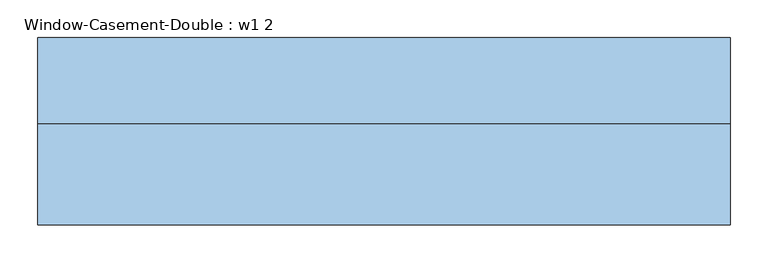
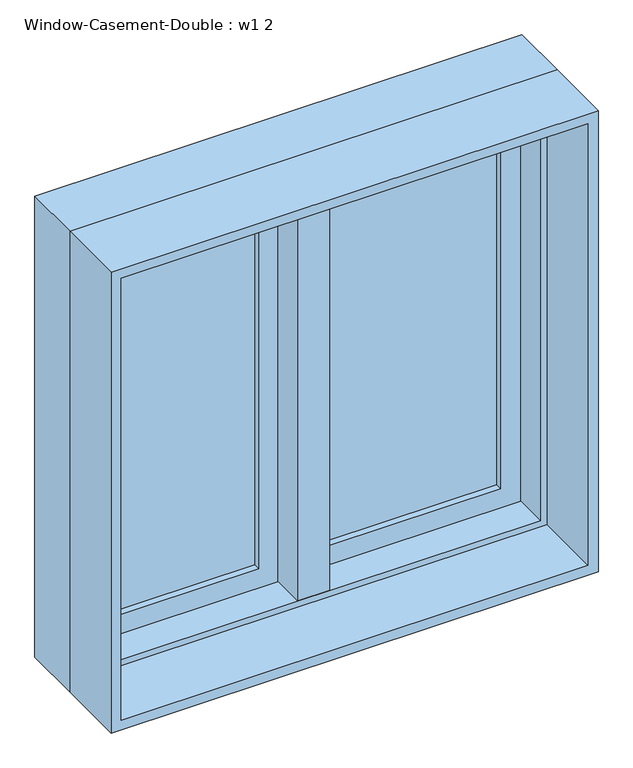
"""IFC4 building model written with IfcOpenShell, lengths in millimetres: window geometry, Window-Casement-Double : w1 2."""

from ifc_helpers import new_model, si_unit, frame, origin, place, context, project, spatial, polyline, outline, extrude, faceted_brep, source, transform, mapped, element, save


def window_casement_double_w1_2_90de19e9(model_context):
    return source(origin(), model_context, "Body", "SolidModel", [
        faceted_brep([(9.525, 133.35, 1816.1), (-9.525, 133.35, 1816.1), (-9.525, 82.55, 1816.1), (9.525, 82.55, 1816.1), (9.525, 133.35, 927.1), (9.525, 82.55, 927.1), (-9.525, 82.55, 927.1), (-9.525, 133.35, 927.1), (-9.525, 82.55, 946.15), (-9.525, 82.55, 1797.05), (-30.1625, 82.55, 946.15), (-30.1625, 82.55, 1797.05), (-30.1625, 19.05, 946.15), (-30.1625, 19.05, 1797.05), (30.1625, 19.05, 946.15), (30.1625, 19.05, 1797.05), (30.1625, 82.55, 946.15), (30.1625, 82.55, 1797.05), (9.525, 82.55, 946.15), (9.525, 82.55, 1797.05)], [[[0, 1, 2, 3]], [[4, 5, 6, 7]], [[1, 0, 4, 7]], [[2, 1, 7, 6, 8, 9]], [[9, 8, 10, 11]], [[11, 10, 12, 13]], [[13, 12, 14, 15]], [[15, 14, 16, 17]], [[17, 16, 18, 19]], [[0, 3, 19, 18, 5, 4]], [[18, 8, 6, 5]], [[9, 19, 3, 2]], [[8, 18, 16, 14, 12, 10]], [[19, 9, 11, 13, 15, 17]]]),
        extrude(outline(polyline([(-66.675, 114.3), (-66.675, 107.95), (-387.35, 107.95), (-387.35, 114.3), (-66.675, 114.3)])), frame((0.0, 0.0, 984.25), z_axis=(0.0, 0.0, 1.0), x_axis=(1.0, 0.0, 0.0)), (0.0, 0.0, 1.0), 774.7),
        extrude(outline(polyline([(-387.35, 95.25), (-387.35, 101.6), (-66.675, 101.6), (-66.675, 95.25), (-387.35, 95.25)])), frame((0.0, 0.0, 984.25), z_axis=(0.0, 0.0, 1.0), x_axis=(1.0, 0.0, 0.0)), (0.0, 0.0, 1.0), 774.7),
        extrude(outline(polyline([(387.35, 114.3), (387.35, 107.95), (66.675, 107.95), (66.675, 114.3), (387.35, 114.3)])), frame((0.0, 0.0, 984.25), z_axis=(0.0, 0.0, 1.0), x_axis=(1.0, 0.0, 0.0)), (0.0, 0.0, 1.0), 774.7),
        extrude(outline(polyline([(66.675, 95.25), (66.675, 101.6), (387.35, 101.6), (387.35, 95.25), (66.675, 95.25)])), frame((0.0, 0.0, 984.25), z_axis=(0.0, 0.0, 1.0), x_axis=(1.0, 0.0, 0.0)), (0.0, 0.0, 1.0), 774.7),
        extrude(outline(polyline([(1816.1, -444.5), (927.1, -444.5), (927.1, -9.525), (1816.1, -9.525), (1816.1, -444.5)]), holes=[polyline([(1758.95, -66.675), (984.25, -66.675), (984.25, -387.35), (1758.95, -387.35), (1758.95, -66.675)])]), frame((0.0, 82.55, 0.0), z_axis=(0.0, 1.0, 0.0), x_axis=(0.0, 0.0, 1.0)), (0.0, 0.0, 1.0), 44.45),
        extrude(outline(polyline([(927.1, 444.5), (1816.1, 444.5), (1816.1, 9.525), (927.1, 9.525), (927.1, 444.5)]), holes=[polyline([(984.25, 66.675), (1758.95, 66.675), (1758.95, 387.35), (984.25, 387.35), (984.25, 66.675)])]), frame((0.0, 82.55, 0.0), z_axis=(0.0, 1.0, 0.0), x_axis=(0.0, 0.0, 1.0)), (0.0, 0.0, 1.0), 44.45),
        extrude(outline(polyline([(1828.8, -457.2), (914.4, -457.2), (914.4, 457.2), (1828.8, 457.2), (1828.8, -457.2)]), holes=[polyline([(1809.75, 438.15), (933.45, 438.15), (933.45, -438.15), (1809.75, -438.15), (1809.75, 438.15)])]), frame((0.0, -114.3, 0.0), z_axis=(0.0, 1.0, 0.0), x_axis=(0.0, 0.0, 1.0)), (0.0, 0.0, 1.0), 133.35),
        faceted_brep([(425.45, 82.55, 1797.05), (425.45, 19.05, 1797.05), (-425.45, 19.05, 1797.05), (-425.45, 82.55, 1797.05), (444.5, 133.35, 1816.1), (444.5, 82.55, 1816.1), (-444.5, 82.55, 1816.1), (-444.5, 133.35, 1816.1), (457.2, 19.05, 1828.8), (457.2, 133.35, 1828.8), (-457.2, 133.35, 1828.8), (-457.2, 19.05, 1828.8), (-425.45, 19.05, 946.15), (-425.45, 82.55, 946.15), (-444.5, 82.55, 927.1), (-444.5, 133.35, 927.1), (-457.2, 133.35, 914.4), (-457.2, 19.05, 914.4), (425.45, 19.05, 946.15), (425.45, 82.55, 946.15), (444.5, 82.55, 927.1), (444.5, 133.35, 927.1), (457.2, 133.35, 914.4), (457.2, 19.05, 914.4)], [[[0, 1, 2, 3]], [[4, 5, 6, 7]], [[8, 9, 10, 11]], [[3, 2, 12, 13]], [[7, 6, 14, 15]], [[11, 10, 16, 17]], [[13, 12, 18, 19]], [[15, 14, 20, 21]], [[17, 16, 22, 23]], [[11, 17, 23, 8], [1, 18, 12, 2]], [[19, 18, 1, 0]], [[5, 20, 14, 6], [3, 13, 19, 0]], [[21, 20, 5, 4]], [[23, 22, 9, 8]], [[9, 22, 16, 10], [7, 15, 21, 4]]]),
    ])


if __name__ == "__main__":
    model = new_model("IFC4")
    model_context = context("Model", 3, world=origin())
    ifc_project = project(units=[si_unit("LENGTHUNIT", "METRE", prefix="MILLI")], contexts=[model_context])
    site = spatial("IfcSite", under=ifc_project)
    building = spatial("IfcBuilding", under=site)
    placement = place(None, origin())
    window_casement_double_w1_2_shape = window_casement_double_w1_2_90de19e9(model_context)
    element("IfcWindow", 1, ObjectType="Window-Casement-Double : w1 2", at=placement, inside=building, context=model_context, shape_type="MappedRepresentation", body=[
        mapped(window_casement_double_w1_2_shape, transform((0.0, 0.0, 0.0), x_axis=(1.0, 0.0, 0.0), y_axis=(0.0, 1.0, 0.0), z_axis=(0.0, 0.0, 1.0))),
    ])
    save(model, "model.ifc")

# Revit data of these elements
# Type "Window-Casement-Double : w1 2"
#   Type Mark = "18"
#   Fire Rating = "0.5h"
#   Assembly Code = "B2020100"
#   Analytic Construction = "Double glazing - domestic"
#   Frame Extension [instance default] = 0' - 0 1/4"
#   Window Inset [instance default] = 0' - 0"
#   Wall Thickness [instance default] = 0' - 6"
#   Interior Wall Closure [instance default] = 0' - 2 1/4"
#   Half Width = 1' - 6"
#   Visual Light Transmittance = 0.81
#   Thermal Resistance (R) = 1.8146 (h·ft²·°F)/BTU
#   Solar Heat Gain Coefficient = 0.76
#   Rough Width = 3' - 0 1/2"
#   Rough Height = 3' - 0 1/2"
#   Height = 3' - 0"
#   Heat Transfer Coefficient (U) = 0.5511 BTU/(h·ft²·°F)
#   Exterior Wall Closure [instance default] = 0' - 1 1/4"
#   Extension Jamb [instance default] = 0' - 2 1/4"
#   Default Sill Height = 3' - 0"
#   Width = 3' - 0"
#   Muntin Visibility = yes
#   Interior Trim Visibility [instance default] = yes
#   Exterior Trim Visibility [instance default] = yes
#   Extension Jamb Visibility [instance default] = yes
#   Muntin Pattern = Muntin Pattern_2x2 : Muntin Pattern_2x2
#   Interior Trim = Trim-Window-Interior-Flat : Picture Frame
#   Interior Frame Material = Wood - Stained
#   Glass Panel Material = Glass
#   Exterior Trim = Trim-Window-Exterior-Flat : with Sill
#   Wall Closure = (empty or 0)
# Element 1 (IfcWindow, "Window-Casement-Double : w1 2")
#   Wall Thickness = 0' - 9"
#   Extension Jamb = 0' - 5 1/4"
#   Materials on its faces: "Wood - Stained", "Glass"
# Materials
#   "Wood - Stained": class "Wood", colour RGB 224 178 126, transparency 0, Cost = 0
#   "Glass": class "Glass", colour RGB 0 128 192, transparency 0.75, Description = "Soda Lime Glass", Cost = 0
